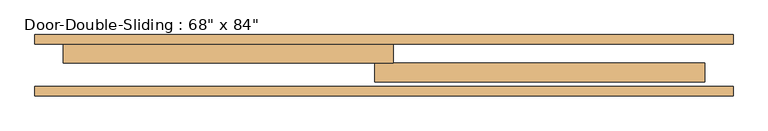
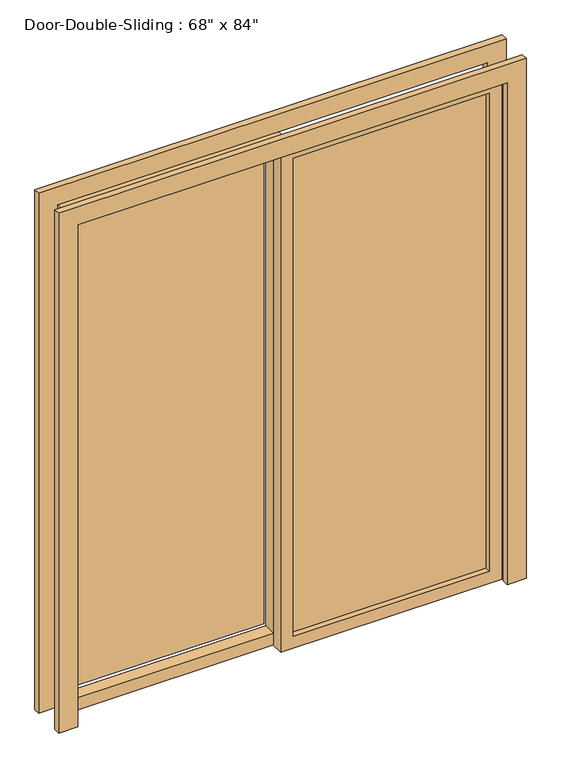
"""IFC4 building model written with IfcOpenShell, lengths in millimetres: door geometry."""

from ifc_helpers import new_model, si_unit, frame, origin, place, context, project, spatial, polyline, outline, extrude, source, transform, mapped, element, save


def door_505787c2(model_context):
    return source(origin(), model_context, "Body", "SweptSolid", [
        extrude(outline(polyline([(0.0, 939.8), (2209.8, 939.8), (2209.8, -939.8), (0.0, -939.8), (0.0, -863.6), (2133.6, -863.6), (2133.6, 863.6), (0.0, 863.6), (0.0, 939.8)])), frame((0.0, 184.15, 0.0), z_axis=(0.0, 1.0, 0.0), x_axis=(0.0, 0.0, 1.0)), (0.0, 0.0, 1.0), 25.4),
        extrude(outline(polyline([(0.0, -939.8), (0.0, -863.6), (2133.6, -863.6), (2133.6, 863.6), (0.0, 863.6), (0.0, 939.8), (2209.8, 939.8), (2209.8, -939.8), (0.0, -939.8)])), frame((0.0, 44.45, 0.0), z_axis=(0.0, 1.0, 0.0), x_axis=(0.0, 0.0, 1.0)), (0.0, 0.0, 1.0), 25.4),
        extrude(outline(polyline([(2133.6, 25.4), (2133.6, -863.6), (0.0, -863.6), (0.0, 25.4), (2133.6, 25.4)]), holes=[polyline([(2082.8, -25.4), (50.8, -25.4), (50.8, -812.8), (2082.8, -812.8), (2082.8, -25.4)])]), frame((0.0, 133.35, 0.0), z_axis=(0.0, 1.0, 0.0), x_axis=(0.0, 0.0, 1.0)), (0.0, 0.0, 1.0), 50.8),
        extrude(outline(polyline([(2133.6, -25.4), (0.0, -25.4), (0.0, 863.6), (2133.6, 863.6), (2133.6, -25.4)]), holes=[polyline([(2082.8, 25.4), (2082.8, 812.8), (50.8, 812.8), (50.8, 25.4), (2082.8, 25.4)])]), frame((0.0, 82.55, 0.0), z_axis=(0.0, 1.0, 0.0), x_axis=(0.0, 0.0, 1.0)), (0.0, 0.0, 1.0), 50.8),
        extrude(outline(polyline([(-25.4, 200.025), (-812.8, 200.025), (-812.8, 206.375), (-25.4, 206.375), (-25.4, 200.025)])), frame((0.0, 0.0, 50.8), z_axis=(0.0, 0.0, 1.0), x_axis=(1.0, 0.0, 0.0)), (0.0, 0.0, 1.0), 2032.0),
        extrude(outline(polyline([(25.4, 111.125), (812.8, 111.125), (812.8, 104.775), (25.4, 104.775), (25.4, 111.125)])), frame((0.0, 0.0, 50.8), z_axis=(0.0, 0.0, 1.0), x_axis=(1.0, 0.0, 0.0)), (0.0, 0.0, 1.0), 2032.0),
    ])


if __name__ == "__main__":
    model = new_model("IFC4")
    model_context = context("Model", 3, world=origin())
    ifc_project = project(units=[si_unit("LENGTHUNIT", "METRE", prefix="MILLI")], contexts=[model_context])
    site = spatial("IfcSite", under=ifc_project)
    building = spatial("IfcBuilding", under=site)
    placement = place(None, origin())
    door_shape = door_505787c2(model_context)
    element("IfcDoor", 1, ObjectType="Door-Double-Sliding : 68\" x 84\"", at=placement, inside=building, context=model_context, shape_type="MappedRepresentation", body=[
        mapped(door_shape, transform((0.0, 0.0, 0.0), x_axis=(1.0, 0.0, 0.0), y_axis=(0.0, 1.0, 0.0), z_axis=(0.0, 0.0, 1.0))),
    ])
    save(model, "model.ifc")

# Revit data of these elements
# Type "Door-Double-Sliding : 68\" x 84\""
#   Type Mark = "14"
#   Construction Type Id = "opn-d45"
#   Assembly Code = "C1020"
#   Analytic Construction = "Wood frame, double glass door "
#   Thickness = 0' - 2"
#   Thermal Resistance (R) = 1.8150 (h·ft²·°F)/BTU
#   Heat Transfer Coefficient (U) = 0.5510 BTU/(h·ft²·°F)
#   Height = 7' - 0"
#   Rail Width = 0' - 2"
#   Stiles = 0' - 2"
#   Trim Projection Ext = 0' - 1"
#   Trim Projection Int = 0' - 1"
#   Trim Width = 0' - 3"
#   Width = 5' - 8"
#   Define Thermal Properties by = 1
#   Glazing = Glass
#   Panel Material = Wood - Birch - Solid Stained Light Low Gloss
#   Trim Material = Paint - Sienna
#   Visual Light Transmittance = 0
#   Solar Heat Gain Coefficient = 0
#   Function = (empty or 0)
#   Wall Closure = (empty or 0)
# Element 1 (IfcDoor, "Door-Double-Sliding : 68\" x 84\"")
#   Materials on its faces: "Paint - Sienna", "Wood - Birch - Solid Stained Light Low Gloss", "Glass"
# Materials
#   "Glass": class "Glass", colour RGB 0 128 192, transparency 0.75, Description = "Soda Lime Glass", Cost = 0
#   "Wood - Birch - Solid Stained Light Low Gloss": class "Wood", colour RGB 210 159 95, transparency 0, Cost = 0
#   "Paint - Sienna": colour RGB 118 70 51, transparency 0, Cost = 0
